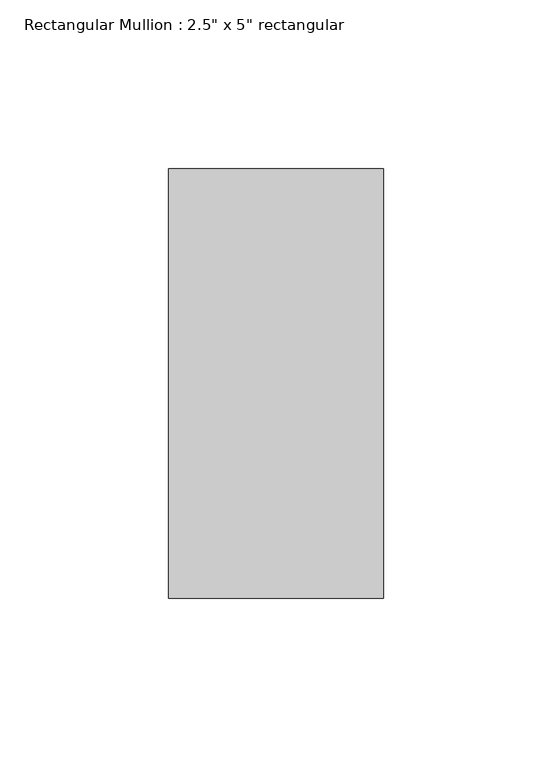
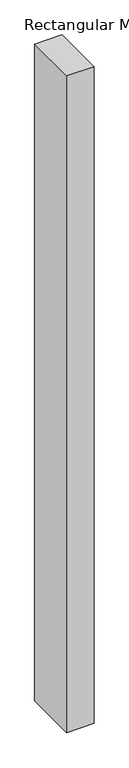
"""IFC4 building model written with IfcOpenShell, lengths in millimetres: member geometry."""

from ifc_helpers import new_model, si_unit, frame, origin, place, context, project, spatial, polyline, outline, extrude, source, transform, mapped, element, save


def member_de6f3820(model_context):
    return source(origin(), model_context, "Body", "SweptSolid", [
        extrude(outline(polyline([(31.75, 63.5), (31.75, -63.5), (-31.75, -63.5), (-31.75, 63.5), (31.75, 63.5)])), frame((0.0, 0.0, -1599.5620987), z_axis=(0.0, 0.0, 1.0), x_axis=(1.0, 0.0, 0.0)), (0.0, 0.0, 1.0), 1599.5620987),
    ])


if __name__ == "__main__":
    model = new_model("IFC4")
    model_context = context("Model", 3, world=origin())
    ifc_project = project(units=[si_unit("LENGTHUNIT", "METRE", prefix="MILLI")], contexts=[model_context])
    site = spatial("IfcSite", under=ifc_project)
    building = spatial("IfcBuilding", under=site)
    placement = place(None, origin())
    member_shape = member_de6f3820(model_context)
    element("IfcMember", 1, ObjectType="Rectangular Mullion : 2.5\" x 5\" rectangular", at=placement, inside=building, context=model_context, shape_type="MappedRepresentation", body=[
        mapped(member_shape, transform((0.0, 0.0, 0.0), x_axis=(1.0, 0.0, 0.0), y_axis=(0.0, 1.0, 0.0), z_axis=(0.0, 0.0, 1.0))),
    ])
    save(model, "model.ifc")

# Revit data of these elements
# Type "Rectangular Mullion : 2.5\" x 5\" rectangular"
#   built-in parameter 1007304 = 0.416667 (stored number, unit not read)
#   built-in parameter 1007301 = 0.104167 (stored number, unit not read)
#   built-in parameter 1007300 = 0.104167 (stored number, unit not read)
# Element 1 (IfcMember, "Rectangular Mullion : 2.5\" x 5\" rectangular")
#   Materials on its faces: "Aluminum"
# Materials
#   "Aluminum": class "Metal", colour RGB 247 247 247, transparency 0, Description = "Aluminum 6061", Cost = 0
